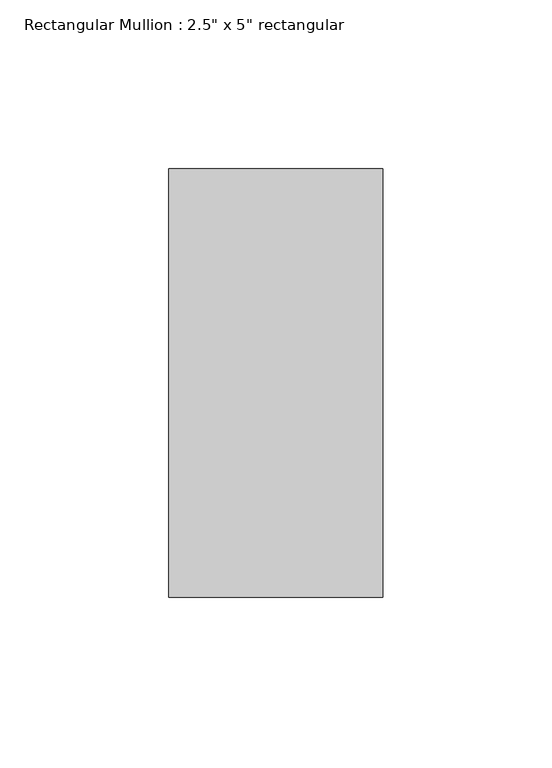
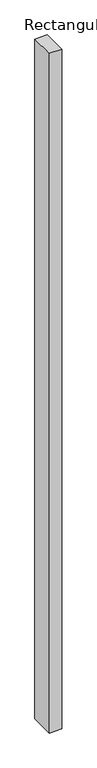
"""IFC4 building model written with IfcOpenShell, lengths in millimetres: member geometry."""

from ifc_helpers import new_model, si_unit, frame, origin, place, context, project, spatial, polyline, outline, extrude, source, transform, mapped, element, save


def member_810865a4(model_context):
    return source(origin(), model_context, "Body", "SweptSolid", [
        extrude(outline(polyline([(31.75, 63.5), (31.75, -63.5), (-31.75, -63.5), (-31.75, 63.5), (31.75, 63.5)])), frame((0.0, 0.0, -3657.6), z_axis=(0.0, 0.0, 1.0), x_axis=(1.0, 0.0, 0.0)), (0.0, 0.0, 1.0), 3657.6),
    ])


if __name__ == "__main__":
    model = new_model("IFC4")
    model_context = context("Model", 3, world=origin())
    ifc_project = project(units=[si_unit("LENGTHUNIT", "METRE", prefix="MILLI")], contexts=[model_context])
    site = spatial("IfcSite", under=ifc_project)
    building = spatial("IfcBuilding", under=site)
    placement = place(None, origin())
    member_shape = member_810865a4(model_context)
    element("IfcMember", 1, ObjectType="Rectangular Mullion : 2.5\" x 5\" rectangular", at=placement, inside=building, context=model_context, shape_type="MappedRepresentation", body=[
        mapped(member_shape, transform((0.0, 0.0, 0.0), x_axis=(1.0, 0.0, 0.0), y_axis=(0.0, 1.0, 0.0), z_axis=(0.0, 0.0, 1.0))),
    ])
    save(model, "model.ifc")

# Revit data of these elements
# Type "Rectangular Mullion : 2.5\" x 5\" rectangular"
#   built-in parameter 1007304 = 0.416667 (stored number, unit not read)
#   built-in parameter 1007301 = 0.104167 (stored number, unit not read)
#   built-in parameter 1007300 = 0.104167 (stored number, unit not read)
# Element 1 (IfcMember, "Rectangular Mullion : 2.5\" x 5\" rectangular")
#   Materials on its faces: "Iron, Ductile"
# Materials
#   "Iron, Ductile": class "Metal", colour RGB 0 0 0, transparency 0, Description = "Ductile cast iron", Cost = 0
